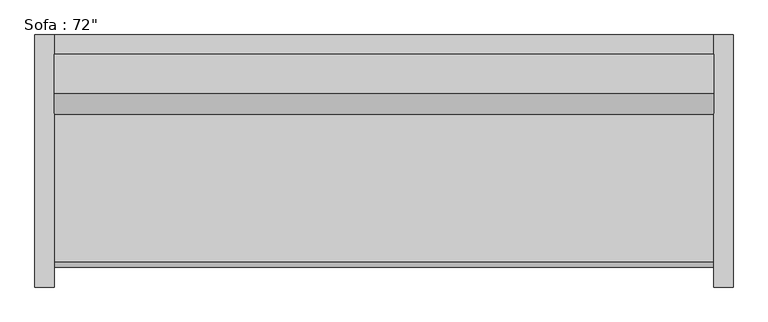
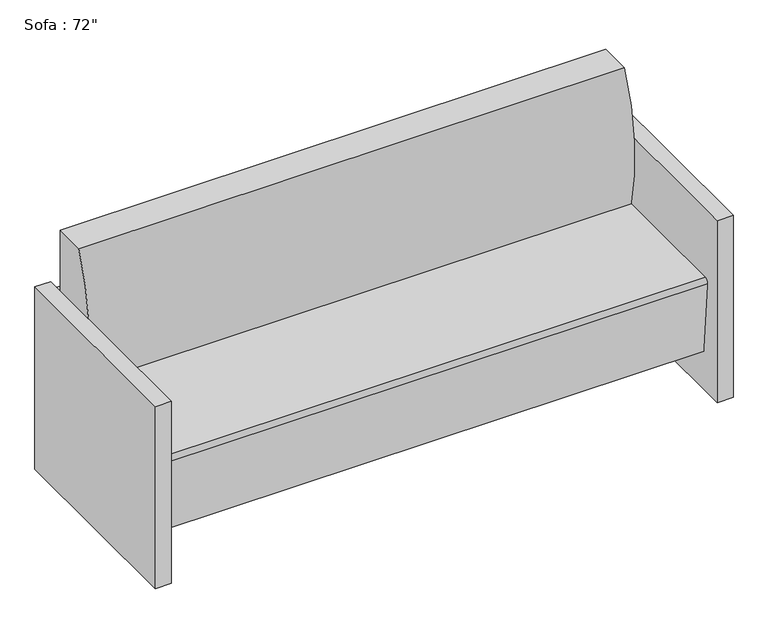
"""IFC4 building model written with IfcOpenShell, lengths in millimetres: furniture geometry."""

from ifc_helpers import new_model, si_unit, point, frame, frame_2d, origin, origin_with_axes, place, context, project, spatial, polyline, circle_curve, trimmed, segment, composite_curve, outline, extrude, source, transform, mapped, element, save


def furniture_a4ffab56(model_context):
    return source(origin(), model_context, "Body", "SweptSolid", [
        extrude(outline(polyline([(-793.2295082, 425.5540984), (-793.2295082, 476.3540984), (933.9704918, 476.3540984), (933.9704918, 425.5540984), (-793.2295082, 425.5540984)])), frame((0.0, 0.0, 457.2), z_axis=(0.0, 0.0, 1.0), x_axis=(1.0, 0.0, 0.0)), (0.0, 0.0, 1.0), 127.0),
        extrude(outline(polyline([(-793.2295082, 425.5540984), (-793.2295082, 476.3540984), (933.9704918, 476.3540984), (933.9704918, 425.5540984), (-793.2295082, 425.5540984)])), frame((0.0, 0.0, 266.7), z_axis=(0.0, 0.0, 1.0), x_axis=(1.0, 0.0, 0.0)), (0.0, 0.0, 1.0), 127.0),
        extrude(outline(polyline([(-793.2295082, 425.5540984), (-793.2295082, 476.3540984), (933.9704918, 476.3540984), (933.9704918, 425.5540984), (-793.2295082, 425.5540984)])), frame((0.0, 0.0, 76.2), z_axis=(0.0, 0.0, 1.0), x_axis=(1.0, 0.0, 0.0)), (0.0, 0.0, 1.0), 127.0),
        extrude(outline(composite_curve([segment(trimmed(circle_curve(frame_2d((926.517198, 542.5300036)), 660.4), [point((286.1764935, 381.0))], [point((323.9540984, 812.8))], False, "CARTESIAN"), True, "CONTINUOUS"), segment(polyline([(323.9540984, 812.8), (425.5540984, 812.8), (425.5540984, 127.9665467), (-111.108343, 127.9665467), (-132.0379563, 367.1931221)]), True, "CONTINUOUS"), segment(trimmed(circle_curve(frame_2d((-119.3862837, 368.3)), 12.7), [point((-132.0379563, 367.1931221))], [point((-119.3862837, 381.0))], False, "CARTESIAN"), True, "CONTINUOUS"), segment(polyline([(-119.3862837, 381.0), (286.1764935, 381.0)]), True, "CONTINUOUS")], self_intersect=False)), frame((-793.2295082, 0.0, 0.0), z_axis=(1.0, 0.0, 0.0), x_axis=(0.0, 1.0, 0.0)), (0.0, 0.0, 1.0), 1727.2),
        extrude(outline(polyline([(-844.0295082, 476.3540984), (-793.2295082, 476.3540984), (-793.2295082, -184.0459016), (-844.0295082, -184.0459016), (-844.0295082, 476.3540984)])), origin_with_axes(), (0.0, 0.0, 1.0), 609.6),
        extrude(outline(polyline([(984.7704918, 476.3540984), (984.7704918, -184.0459016), (933.9704918, -184.0459016), (933.9704918, 476.3540984), (984.7704918, 476.3540984)])), origin_with_axes(), (0.0, 0.0, 1.0), 609.6),
    ])


if __name__ == "__main__":
    model = new_model("IFC4")
    model_context = context("Model", 3, world=origin())
    ifc_project = project(units=[si_unit("LENGTHUNIT", "METRE", prefix="MILLI")], contexts=[model_context])
    site = spatial("IfcSite", under=ifc_project)
    building = spatial("IfcBuilding", under=site)
    placement = place(None, origin())
    furniture_shape = furniture_a4ffab56(model_context)
    element("IfcFurniture", 1, ObjectType="Sofa : 72\"", at=placement, inside=building, context=model_context, shape_type="MappedRepresentation", body=[
        mapped(furniture_shape, transform((0.0, 0.0, 0.0), x_axis=(1.0, 0.0, 0.0), y_axis=(0.0, 1.0, 0.0), z_axis=(0.0, 0.0, 1.0))),
    ])
    save(model, "model.ifc")

# Revit data of these elements
# Type "Sofa : 72\""
#   Assembly Code = "E2020200"
#   Width = 6' - 0"
#   Seat Material = Leather - Black
#   Frame Material = Carpet (2)
#   Default Elevation = 0
# Element 1 (IfcFurniture, "Sofa : 72\"")
#   Materials on its faces: "Cherry", "Carpet (2)", "Leather - Black"
# Materials
#   "Leather - Black": class "Generic", colour RGB 40 40 40, transparency 0, Cost = 0
#   "Carpet (2)": class "Carpet", colour RGB 0 0 0, transparency 0, Description = "Interior finish"
#   "Cherry": class "Wood", colour RGB 226 177 128, transparency 0, Description = "Prunus Serotina", Cost = 0
